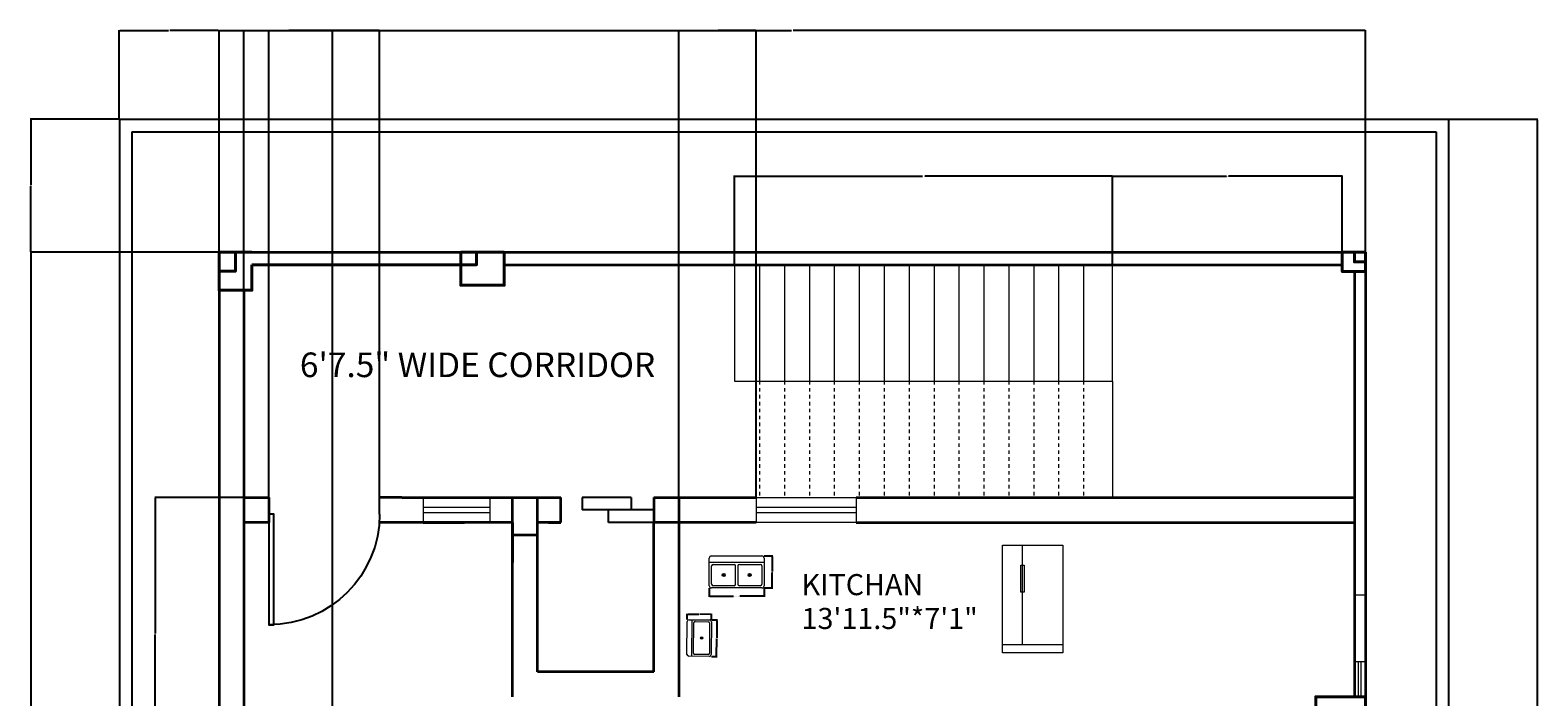
# Model space of a CAD drawing. Units: inches. Extents: x -1085 to 1941, y 1514 to 2348.
# Tile 9 of 9: x 1397 to 1941, y 1974 to 2214. Entities that reach past the tile are written whole.
import ezdxf

# ---------------------------------------------------------------- set-up
doc = ezdxf.new("R2010")
doc.units = ezdxf.units.IN
doc.linetypes.add('JIS_02_1.2', pattern=[2.5, 1.25, -1.25])
for name, color, linetype, lineweight in [('A-ANNO-DIMS', 2, 'Continuous', 18), ('A-AREA-IDEN', 7, 'Continuous', 25), ('A-COLS', 7, 'Continuous', 40), ('A-DOOR', 4, 'Continuous', 25), ('A-EQPM', 9, 'Continuous', 18), ('A-FLOR-FIXT', 9, 'Continuous', 18), ('A-FLOR-STRS', 1, 'Continuous', 18), ('A-FLOR-STRS-HIDN', 1, 'JIS_02_1.2', 18), ('A-GLAZ', 180, 'Continuous', 18), ('A-WALL', 7, 'Continuous', 35), ('C-PROP', 8, 'Continuous', 25)]:
    doc.layers.add(name, color=color, linetype=linetype, lineweight=lineweight)
doc.styles.get("Standard").update_dxf_attribs({"font": 'arial.ttf'})
doc.dimstyles.get("Standard").update_dxf_attribs({"dimtxt": 0.18, "dimasz": 0.18, "dimexe": 0.18, "dimexo": 0.0625, "dimgap": 0.09, "dimtad": 0, "dimtih": 1, "dimtoh": 1, "dimdec": 4, "dimzin": 0, "dimdsep": 46, "dimtxsty": 'Standard', "dimcen": 0.09, "dimadec": 0, "dimazin": 0, "dimtfac": 1, "dimtdec": 4, "dimtofl": 0, "dimtmove": 0, "dimatfit": 3, "dimfxl": 1, "dimtolj": 1, "dimtzin": 0, "dimarcsym": 0})

# ---------------------------------------------------------------- blocks, each defined once
blk = doc.blocks.new('*U2')
for p, q in [((0, 0), (0, -6)), ((40, 0), (40, -6))]:
    blk.add_line(p, q)
blk.add_lwpolyline([(0, 0), (0, 40), (1.75, 40), (1.75, 0)], close=True)
blk.add_arc((0, 0), 40, 0, 90)
blk = doc.blocks.new('Refrigerator-2 door - 36 in front')
for p, q in [((12, 5), (12, 64)), ((0, 5), (36, 5))]:
    blk.add_line(p, q)
for points in [[(0, 0), (0, 64), (36, 64), (36, 0)], [(11, 36), (11, 52), (13, 52), (13, 36)]]:
    blk.add_lwpolyline(points, close=True)
blk = doc.blocks.new('Sink-double - 36 in top')
for p, q in [((-18, -4), (18, -4)), ((-0.75, -18.5), (-0.75, -6.5)), ((0.75, -6.5), (0.75, -18.5))]:
    blk.add_line(p, q)
for points in [[(-16.5, 0), (16.5, 0)], [(-18, -19.5), (-18, -1.5)], [(-16.5, -18.5), (-16.5, -6.5)], [(-15.5, -5.5), (-1.75, -5.5)], [(1.75, -5.5), (15.5, -5.5)], [(16.5, -6.5), (16.5, -18.5)], [(18, -1.5), (18, -19.5)], [(-1.75, -19.5), (-15.5, -19.5)], [(15.5, -19.5), (1.75, -19.5)], [(16.5, -21), (-16.5, -21)]]:
    blk.add_lwpolyline(points)
for centre, radius in [((-8.5, -12.5), 1), ((-8.5, -12.5), 0.5), ((8.5, -12.5), 1), ((8.5, -12.5), 0.5)]:
    blk.add_circle(centre, radius)
for centre, radius, start, end in [((-16.5, -1.5), 1.5, 90, 180), ((16.5, -1.5), 1.5, 0, 90), ((-15.5, -6.5), 1, 90, 180), ((-1.75, -6.5), 1, 0, 90), ((1.75, -6.5), 1, 90, 180), ((15.5, -6.5), 1, 0, 90), ((-16.5, -19.5), 1.5, 180, 270), ((-15.5, -18.5), 1, 180, 270), ((-1.75, -18.5), 1, 270, 0), ((1.75, -18.5), 1, 180, 270), ((15.5, -18.5), 1, 270, 0), ((16.5, -19.5), 1.5, 270, 0)]:
    blk.add_arc(centre, radius, start, end)
blk = doc.blocks.new('Sink-single - 30 in top')
blk.add_line((-15, -3.999996), (15, -3.999996))
for points in [[(-13.5, 0), (13.5, 0)], [(-15, -18.499996), (-15, -1.5)], [(-13.5, -17.499996), (-13.5, -6.499996)], [(-12.5, -5.499996), (12.5, -5.499996)], [(13.5, -6.499996), (13.5, -17.499996)], [(15, -1.5), (15, -18.499996)], [(13.5, -19.999996), (-13.5, -19.999996)], [(12.5, -18.499996), (-12.5, -18.499996)]]:
    blk.add_lwpolyline(points)
for radius in [1, 0.5]:
    blk.add_circle((0, -11.999996), radius)
for centre, radius, start, end in [((-13.5, -1.5), 1.5, 90, 180), ((-12.5, -6.499996), 1, 90, 180), ((12.5, -6.499996), 1, 0, 90), ((13.5, -1.5), 1.5, 0, 90), ((-13.5, -18.499996), 1.5, 180, 270), ((-12.5, -17.499996), 1, 180, 270), ((12.5, -17.499996), 1, 270, 0), ((13.5, -18.499996), 1.5, 270, 0)]:
    blk.add_arc(centre, radius, start, end)
blk = doc.blocks.new('WIN-36-9')
for p, q in [((0, 9), (0, 0)), ((0, 5.5), (36, 5.5)), ((36, 9), (36, 0)), ((36, 3.5), (0, 3.5))]:
    blk.add_line(p, q)
blk = doc.blocks.new('*D70')
at = {"layer": 'A-ANNO-DIMS', "color": 0, "lineweight": -2, "transparency": 16777216}
for p, q in [((1642.11, 2013.01), (1642.11, 2009.92)), ((1642.29, 2010.1), (1650.92, 2010.1)), ((1661.73, 2010.1), (1653.11, 2010.1)), ((1661.91, 2013.01), (1661.91, 2009.92))]:
    blk.add_line(p, q, dxfattribs=at)
at = {"layer": 'A-ANNO-DIMS', "color": 0, "transparency": 16777216}
for points in [[(1642.29, 2010.13), (1642.29, 2010.07), (1642.11, 2010.1)], [(1661.73, 2010.13), (1661.73, 2010.07), (1661.91, 2010.1)]]:
    blk.add_solid(points, dxfattribs=at)
at = {"layer": 'Defpoints', "color": 0, "transparency": 16777216}
for p in [(1642.11, 2013.07), (1661.91, 2013.07), (1661.91, 2010.1)]:
    blk.add_point(p, dxfattribs=at)
at = {"layer": 'A-ANNO-DIMS', "color": 0, "transparency": 16777216, "insert": (1652.01, 2010.1), "char_height": 0.18, "attachment_point": 5}
blk.add_mtext('\\A1;DOUBLE SINK 20', dxfattribs=at)
blk = doc.blocks.new('*D71')
at = {"layer": 'A-ANNO-DIMS', "color": 0, "lineweight": -2, "transparency": 16777216}
for p, q in [((1661.97, 2024.62), (1665.06, 2024.62)), ((1664.88, 2024.44), (1664.88, 2019.03)), ((1664.88, 2013.25), (1664.88, 2018.67)), ((1661.97, 2013.07), (1665.06, 2013.07))]:
    blk.add_line(p, q, dxfattribs=at)
at = {"layer": 'A-ANNO-DIMS', "color": 0, "transparency": 16777216}
for points in [[(1664.85, 2024.44), (1664.91, 2024.44), (1664.88, 2024.62)], [(1664.85, 2013.25), (1664.91, 2013.25), (1664.88, 2013.07)]]:
    blk.add_solid(points, dxfattribs=at)
at = {"layer": 'Defpoints', "color": 0, "transparency": 16777216}
for p in [(1661.91, 2024.62), (1664.88, 2024.62), (1661.91, 2013.07)]:
    blk.add_point(p, dxfattribs=at)
at = {"layer": 'A-ANNO-DIMS', "color": 0, "transparency": 16777216, "insert": (1664.88, 2018.85), "char_height": 0.18, "attachment_point": 5}
blk.add_mtext('\\A1;12', dxfattribs=at)
blk = doc.blocks.new('*D72')
at = {"layer": 'A-ANNO-DIMS', "color": 0, "lineweight": -2, "transparency": 16777216}
for p, q in [((1642.98, 2001.55), (1645.08, 2001.53)), ((1644.89, 2001.36), (1644.84, 1995.13)), ((1644.78, 1988.54), (1644.84, 1994.77)), ((1642.87, 1988.38), (1644.96, 1988.36))]:
    blk.add_line(p, q, dxfattribs=at)
at = {"layer": 'A-ANNO-DIMS', "color": 0, "transparency": 16777216}
for points in [[(1644.86, 2001.36), (1644.92, 2001.36), (1644.9, 2001.54)], [(1644.75, 1988.54), (1644.81, 1988.54), (1644.78, 1988.36)]]:
    blk.add_solid(points, dxfattribs=at)
at = {"layer": 'Defpoints', "color": 0, "transparency": 16777216}
for p in [(1642.92, 2001.55), (1644.9, 2001.54), (1642.81, 1988.38)]:
    blk.add_point(p, dxfattribs=at)
at = {"layer": 'A-ANNO-DIMS', "color": 0, "transparency": 16777216, "insert": (1644.84, 1994.95), "char_height": 0.18, "attachment_point": 5}
blk.add_mtext('\\A1;SINGLE SINK 13', dxfattribs=at)
blk = doc.blocks.new('*D73')
at = {"layer": 'A-ANNO-DIMS', "color": 0, "lineweight": -2, "transparency": 16777216}
for p, q in [((1634.14, 2001.69), (1634.16, 2003.79)), ((1634.33, 2003.6), (1638.4, 2003.57)), ((1642.76, 2003.53), (1638.69, 2003.57)), ((1642.92, 2001.62), (1642.94, 2003.71))]:
    blk.add_line(p, q, dxfattribs=at)
at = {"layer": 'A-ANNO-DIMS', "color": 0, "transparency": 16777216}
for points in [[(1634.33, 2003.63), (1634.33, 2003.57), (1634.15, 2003.61)], [(1642.76, 2003.56), (1642.76, 2003.5), (1642.94, 2003.53)]]:
    blk.add_solid(points, dxfattribs=at)
at = {"layer": 'Defpoints', "color": 0, "transparency": 16777216}
for p in [(1634.15, 2003.61), (1634.14, 2001.63), (1642.92, 2001.55)]:
    blk.add_point(p, dxfattribs=at)
at = {"layer": 'A-ANNO-DIMS', "color": 0, "transparency": 16777216, "insert": (1638.55, 2003.57), "char_height": 0.18, "attachment_point": 5}
blk.add_mtext('\\A1;9', dxfattribs=at)
blk = doc.blocks.new('*D75')
at = {"layer": 'A-ANNO-DIMS', "color": 0, "lineweight": -2, "transparency": 16777216}
for p, q in [((1909.16, 2182.24), (1941.27, 2182.24)), ((1941.09, 2182.06), (1941.09, 1864.42)), ((1941.09, 1546.42), (1941.09, 1864.06)), ((1909.16, 1546.24), (1941.27, 1546.24))]:
    blk.add_line(p, q, dxfattribs=at)
at = {"layer": 'A-ANNO-DIMS', "color": 0, "transparency": 16777216}
for points in [[(1941.06, 2182.06), (1941.12, 2182.06), (1941.09, 2182.24)], [(1941.06, 1546.42), (1941.12, 1546.42), (1941.09, 1546.24)]]:
    blk.add_solid(points, dxfattribs=at)
at = {"layer": 'Defpoints', "color": 0, "transparency": 16777216}
for p in [(1909.09, 2182.24), (1941.09, 2182.24), (1909.09, 1546.24)]:
    blk.add_point(p, dxfattribs=at)
at = {"layer": 'A-ANNO-DIMS', "color": 0, "transparency": 16777216, "insert": (1941.09, 1864.24), "char_height": 0.18, "attachment_point": 5}
blk.add_mtext('\\A1;636', dxfattribs=at)
blk = doc.blocks.new('*D76')
at = {"layer": 'A-ANNO-DIMS', "color": 0, "lineweight": -2, "transparency": 16777216}
for p, q in [((1465.09, 2134.3), (1465.09, 2214.42)), ((1465.27, 2214.24), (1671.8, 2214.24)), ((1878.91, 2214.24), (1672.39, 2214.24)), ((1879.09, 2134.3), (1879.09, 2214.42))]:
    blk.add_line(p, q, dxfattribs=at)
at = {"layer": 'A-ANNO-DIMS', "color": 0, "transparency": 16777216}
for points in [[(1465.27, 2214.27), (1465.27, 2214.21), (1465.09, 2214.24)], [(1878.91, 2214.27), (1878.91, 2214.21), (1879.09, 2214.24)]]:
    blk.add_solid(points, dxfattribs=at)
at = {"layer": 'Defpoints', "color": 0, "transparency": 16777216}
for p in [(1879.09, 2214.24), (1465.09, 2134.24), (1879.09, 2134.24)]:
    blk.add_point(p, dxfattribs=at)
at = {"layer": 'A-ANNO-DIMS', "color": 0, "transparency": 16777216, "insert": (1672.09, 2214.24), "char_height": 0.18, "attachment_point": 5}
blk.add_mtext('\\A1;414', dxfattribs=at)
blk = doc.blocks.new('*D77')
at = {"layer": 'A-ANNO-DIMS', "color": 0, "lineweight": -2, "transparency": 16777216}
for p, q in [((1465.03, 2134.24), (1396.91, 2134.24)), ((1397.09, 2134.06), (1397.09, 1855.42)), ((1397.09, 1576.42), (1397.09, 1855.06)), ((1465.03, 1576.24), (1396.91, 1576.24))]:
    blk.add_line(p, q, dxfattribs=at)
at = {"layer": 'A-ANNO-DIMS', "color": 0, "transparency": 16777216}
for points in [[(1397.06, 2134.06), (1397.12, 2134.06), (1397.09, 2134.24)], [(1397.06, 1576.42), (1397.12, 1576.42), (1397.09, 1576.24)]]:
    blk.add_solid(points, dxfattribs=at)
at = {"layer": 'Defpoints', "color": 0, "transparency": 16777216}
for p in [(1397.09, 2134.24), (1465.09, 2134.24), (1465.09, 1576.24)]:
    blk.add_point(p, dxfattribs=at)
at = {"layer": 'A-ANNO-DIMS', "color": 0, "transparency": 16777216, "insert": (1397.09, 1855.24), "char_height": 0.18, "attachment_point": 5}
blk.add_mtext('\\A1;558', dxfattribs=at)
blk = doc.blocks.new('*D78')
at = {"layer": 'A-ANNO-DIMS', "color": 0, "lineweight": -2, "transparency": 16777216}
for p, q in [((1429.09, 2182.3), (1429.09, 2214.42)), ((1429.27, 2214.24), (1446.88, 2214.24)), ((1464.91, 2214.24), (1447.31, 2214.24)), ((1465.09, 2134.3), (1465.09, 2214.42))]:
    blk.add_line(p, q, dxfattribs=at)
at = {"layer": 'A-ANNO-DIMS', "color": 0, "transparency": 16777216}
for points in [[(1429.27, 2214.27), (1429.27, 2214.21), (1429.09, 2214.24)], [(1464.91, 2214.27), (1464.91, 2214.21), (1465.09, 2214.24)]]:
    blk.add_solid(points, dxfattribs=at)
at = {"layer": 'Defpoints', "color": 0, "transparency": 16777216}
for p in [(1465.09, 2214.24), (1429.09, 2182.24), (1465.09, 2134.24)]:
    blk.add_point(p, dxfattribs=at)
at = {"layer": 'A-ANNO-DIMS', "color": 0, "transparency": 16777216, "insert": (1447.09, 2214.24), "char_height": 0.18, "attachment_point": 5}
blk.add_mtext('\\A1;36', dxfattribs=at)
blk = doc.blocks.new('*D79')
at = {"layer": 'A-ANNO-DIMS', "color": 0, "lineweight": -2, "transparency": 16777216}
for p, q in [((1429.03, 2182.24), (1396.91, 2182.24)), ((1397.09, 2182.06), (1397.09, 2158.42)), ((1397.09, 2134.42), (1397.09, 2158.06)), ((1465.03, 2134.24), (1396.91, 2134.24))]:
    blk.add_line(p, q, dxfattribs=at)
at = {"layer": 'A-ANNO-DIMS', "color": 0, "transparency": 16777216}
for points in [[(1397.06, 2182.06), (1397.12, 2182.06), (1397.09, 2182.24)], [(1397.06, 2134.42), (1397.12, 2134.42), (1397.09, 2134.24)]]:
    blk.add_solid(points, dxfattribs=at)
at = {"layer": 'Defpoints', "color": 0, "transparency": 16777216}
for p in [(1429.09, 2182.24), (1397.09, 2134.24), (1465.09, 2134.24)]:
    blk.add_point(p, dxfattribs=at)
at = {"layer": 'A-ANNO-DIMS', "color": 0, "transparency": 16777216, "insert": (1397.09, 2158.24), "char_height": 0.18, "attachment_point": 5}
blk.add_mtext('\\A1;48', dxfattribs=at)
blk = doc.blocks.new('*D80')
at = {"layer": 'A-ANNO-DIMS', "color": 0, "lineweight": -2, "transparency": 16777216}
for p, q in [((1483.09, 2045.8), (1483.09, 2214.42)), ((1483.27, 2214.24), (1502.87, 2214.24)), ((1522.91, 2214.24), (1503.32, 2214.24)), ((1523.09, 2045.8), (1523.09, 2214.42))]:
    blk.add_line(p, q, dxfattribs=at)
at = {"layer": 'A-ANNO-DIMS', "color": 0, "transparency": 16777216}
for points in [[(1483.27, 2214.27), (1483.27, 2214.21), (1483.09, 2214.24)], [(1522.91, 2214.27), (1522.91, 2214.21), (1523.09, 2214.24)]]:
    blk.add_solid(points, dxfattribs=at)
at = {"layer": 'Defpoints', "color": 0, "transparency": 16777216}
for p in [(1523.09, 2214.24), (1483.09, 2045.74), (1523.09, 2045.74)]:
    blk.add_point(p, dxfattribs=at)
at = {"layer": 'A-ANNO-DIMS', "color": 0, "transparency": 16777216, "insert": (1503.09, 2214.24), "char_height": 0.18, "attachment_point": 5}
blk.add_mtext('\\A1;40', dxfattribs=at)
blk = doc.blocks.new('*D84')
at = {"layer": 'A-ANNO-DIMS', "color": 0, "lineweight": -2, "transparency": 16777216}
for p, q in [((1474.09, 1651.3), (1474.09, 2214.42)), ((1474.27, 2214.24), (1489.88, 2214.24)), ((1505.91, 2214.24), (1490.31, 2214.24)), ((1506.09, 1651.3), (1506.09, 2214.42))]:
    blk.add_line(p, q, dxfattribs=at)
at = {"layer": 'A-ANNO-DIMS', "color": 0, "transparency": 16777216}
for points in [[(1474.27, 2214.27), (1474.27, 2214.21), (1474.09, 2214.24)], [(1505.91, 2214.27), (1505.91, 2214.21), (1506.09, 2214.24)]]:
    blk.add_solid(points, dxfattribs=at)
at = {"layer": 'Defpoints', "color": 0, "transparency": 16777216}
for p in [(1506.09, 2214.24), (1474.09, 1651.24), (1506.09, 1651.24)]:
    blk.add_point(p, dxfattribs=at)
at = {"layer": 'A-ANNO-DIMS', "color": 0, "transparency": 16777216, "insert": (1490.09, 2214.24), "char_height": 0.18, "attachment_point": 5}
blk.add_mtext('\\A1;32', dxfattribs=at)
blk = doc.blocks.new('*D90')
at = {"layer": 'A-ANNO-DIMS', "color": 0, "lineweight": -2, "transparency": 16777216}
for p, q in [((1474.03, 2045.74), (1441.91, 2045.74)), ((1442.09, 2045.56), (1442.09, 1996.67)), ((1442.09, 1947.42), (1442.09, 1996.31)), ((1474.03, 1947.24), (1441.91, 1947.24))]:
    blk.add_line(p, q, dxfattribs=at)
at = {"layer": 'A-ANNO-DIMS', "color": 0, "transparency": 16777216}
for points in [[(1442.06, 2045.56), (1442.12, 2045.56), (1442.09, 2045.74)], [(1442.06, 1947.42), (1442.12, 1947.42), (1442.09, 1947.24)]]:
    blk.add_solid(points, dxfattribs=at)
at = {"layer": 'Defpoints', "color": 0, "transparency": 16777216}
for p in [(1442.09, 2045.74), (1474.09, 2045.74), (1474.09, 1947.24)]:
    blk.add_point(p, dxfattribs=at)
at = {"layer": 'A-ANNO-DIMS', "color": 0, "transparency": 16777216, "insert": (1442.09, 1996.49), "char_height": 0.18, "attachment_point": 5}
blk.add_mtext('\\A1;98.5', dxfattribs=at)
blk = doc.blocks.new('*D91')
at = {"layer": 'A-ANNO-DIMS', "color": 0, "lineweight": -2, "transparency": 16777216}
for p, q in [((1631.09, 2045.8), (1631.09, 2214.42)), ((1631.27, 2214.24), (1644.87, 2214.24)), ((1658.91, 2214.24), (1645.32, 2214.24)), ((1659.09, 2045.8), (1659.09, 2214.42))]:
    blk.add_line(p, q, dxfattribs=at)
at = {"layer": 'A-ANNO-DIMS', "color": 0, "transparency": 16777216}
for points in [[(1631.27, 2214.27), (1631.27, 2214.21), (1631.09, 2214.24)], [(1658.91, 2214.27), (1658.91, 2214.21), (1659.09, 2214.24)]]:
    blk.add_solid(points, dxfattribs=at)
at = {"layer": 'Defpoints', "color": 0, "transparency": 16777216}
for p in [(1659.09, 2214.24), (1631.09, 2045.74), (1659.09, 2045.74)]:
    blk.add_point(p, dxfattribs=at)
at = {"layer": 'A-ANNO-DIMS', "color": 0, "transparency": 16777216, "insert": (1645.09, 2214.24), "char_height": 0.18, "attachment_point": 5}
blk.add_mtext('\\A1;28', dxfattribs=at)
blk = doc.blocks.new('*D92')
at = {"layer": 'A-ANNO-DIMS', "color": 0, "lineweight": -2, "transparency": 16777216}
for p, q in [((1651.26, 2129.8), (1651.26, 2161.92)), ((1651.44, 2161.74), (1719.05, 2161.74)), ((1787.57, 2161.74), (1719.96, 2161.74)), ((1787.75, 2129.8), (1787.75, 2161.92))]:
    blk.add_line(p, q, dxfattribs=at)
at = {"layer": 'A-ANNO-DIMS', "color": 0, "transparency": 16777216}
for points in [[(1651.44, 2161.77), (1651.44, 2161.71), (1651.26, 2161.74)], [(1787.57, 2161.77), (1787.57, 2161.71), (1787.75, 2161.74)]]:
    blk.add_solid(points, dxfattribs=at)
at = {"layer": 'Defpoints', "color": 0, "transparency": 16777216}
for p in [(1787.75, 2161.74), (1651.26, 2129.74), (1787.75, 2129.74)]:
    blk.add_point(p, dxfattribs=at)
at = {"layer": 'A-ANNO-DIMS', "color": 0, "transparency": 16777216, "insert": (1719.5, 2161.74), "char_height": 0.18, "attachment_point": 5}
blk.add_mtext('\\A1;136.48', dxfattribs=at)
blk = doc.blocks.new('*D93')
at = {"layer": 'A-ANNO-DIMS', "color": 0, "lineweight": -2, "transparency": 16777216}
for p, q in [((1787.75, 2129.8), (1787.75, 2161.92)), ((1787.93, 2161.74), (1828.82, 2161.74)), ((1870.5, 2161.74), (1829.61, 2161.74)), ((1870.68, 2129.8), (1870.68, 2161.92))]:
    blk.add_line(p, q, dxfattribs=at)
at = {"layer": 'A-ANNO-DIMS', "color": 0, "transparency": 16777216}
for points in [[(1787.93, 2161.77), (1787.93, 2161.71), (1787.75, 2161.74)], [(1870.5, 2161.77), (1870.5, 2161.71), (1870.68, 2161.74)]]:
    blk.add_solid(points, dxfattribs=at)
at = {"layer": 'Defpoints', "color": 0, "transparency": 16777216}
for p in [(1870.68, 2161.74), (1787.75, 2129.74), (1870.68, 2129.74)]:
    blk.add_point(p, dxfattribs=at)
at = {"layer": 'A-ANNO-DIMS', "color": 0, "transparency": 16777216, "insert": (1829.21, 2161.74), "char_height": 0.18, "attachment_point": 5}
blk.add_mtext('\\A1;82.93', dxfattribs=at)

msp = doc.modelspace()

# ---------------------------------------------------------------- linework, layer by layer
at = {"layer": 'A-COLS'}
msp.add_lwpolyline([(1476.9484, 2129.7392), (1476.9484, 2120.553), (1465.0949, 2120.553), (1465.0949, 2134.2392), (1476.9484, 2134.2392)], dxfattribs=at)
for points in [[(1465.0949, 2134.2392), (1471.0216, 2134.2392), (1471.0216, 2127.3961), (1465.0949, 2127.3961)], [(1552.4003, 2134.2392), (1568.1037, 2134.2392), (1568.1037, 2122.3334), (1552.4003, 2122.3334)], [(1552.4003, 2134.2392), (1558.0949, 2134.2392), (1558.0949, 2129.7392), (1552.4003, 2129.7392)], [(1879.0949, 2134.2392), (1870.6776, 2134.2392), (1870.6776, 2127.2968), (1879.0949, 2127.2968)], [(1879.0949, 2134.2392), (1875.0637, 2134.2392), (1875.0637, 2130.768), (1879.0949, 2130.768)], [(1879.0949, 1973.8073), (1879.0949, 1961.8073), (1861.0949, 1961.8073), (1861.0949, 1973.8073)]]:
    msp.add_lwpolyline(points, close=True, dxfattribs=at)
at = {"layer": 'A-DOOR'}
for p, q in [((1613.8856, 2045.7392), (1596.2389, 2045.7392)), ((1596.2389, 2045.7392), (1596.2389, 2041.2392)), ((1613.8856, 2045.7392), (1613.8856, 2041.2392)), ((1613.8856, 2041.2392), (1596.2389, 2041.2392)), ((1622.0949, 2041.2392), (1605.6763, 2041.2392)), ((1605.6763, 2036.7392), (1605.6763, 2041.2392)), ((1622.0949, 2036.7392), (1605.6763, 2036.7392))]:
    msp.add_line(p, q, dxfattribs=at)
at = {"layer": 'A-FLOR-STRS'}
for p, q in [((1651.2617, 2129.7392), (1651.2617, 2087.7392)), ((1660.2617, 2129.7392), (1660.2617, 2087.7392)), ((1669.2617, 2129.7392), (1669.2617, 2087.7392)), ((1678.2617, 2129.7392), (1678.2617, 2087.7392)), ((1687.2617, 2129.7392), (1687.2617, 2087.7392)), ((1696.2617, 2129.7392), (1696.2617, 2087.7392)), ((1705.2617, 2129.7392), (1705.2617, 2087.7392)), ((1714.2617, 2129.7392), (1714.2617, 2087.7392)), ((1723.2617, 2129.7392), (1723.2617, 2087.7392)), ((1732.2617, 2129.7392), (1732.2617, 2087.7392)), ((1741.2617, 2129.7392), (1741.2617, 2087.7392)), ((1750.2617, 2129.7392), (1750.2617, 2087.7392)), ((1759.2617, 2129.7392), (1759.2617, 2087.7392)), ((1768.2617, 2129.7392), (1768.2617, 2087.7392)), ((1777.2617, 2129.7392), (1777.2617, 2087.7392)), ((1787.7455, 2087.7392), (1787.7455, 2129.7392)), ((1651.2617, 2087.7392), (1787.7455, 2087.7392)), ((1787.7455, 2087.7392), (1787.7455, 2045.7392))]:
    msp.add_line(p, q, dxfattribs=at)
at = {"layer": 'A-FLOR-STRS-HIDN'}
for p, q in [((1660.2617, 2087.7392), (1660.2617, 2045.7392)), ((1669.2617, 2087.7392), (1669.2617, 2045.7392)), ((1678.2617, 2087.7392), (1678.2617, 2045.7392)), ((1687.2617, 2087.7392), (1687.2617, 2045.7392)), ((1696.2617, 2087.7392), (1696.2617, 2045.7392)), ((1705.2617, 2087.7392), (1705.2617, 2045.7392)), ((1705.2617, 2087.7392), (1705.2617, 2045.7392)), ((1714.2617, 2087.7392), (1714.2617, 2045.7392)), ((1723.2617, 2087.7392), (1723.2617, 2045.7392)), ((1732.2617, 2087.7392), (1732.2617, 2045.7392)), ((1741.2617, 2087.7392), (1741.2617, 2045.7392)), ((1750.2617, 2087.7392), (1750.2617, 2045.7392)), ((1759.2617, 2087.7392), (1759.2617, 2045.7392)), ((1768.2617, 2087.7392), (1768.2617, 2045.7392)), ((1777.2617, 2087.7392), (1777.2617, 2045.7392))]:
    msp.add_line(p, q, dxfattribs=at)
at = {"layer": 'A-GLAZ'}
for p, q in [((1538.837, 2045.7392), (1538.837, 2036.7392)), ((1538.837, 2042.2392), (1552.5949, 2042.2392)), ((1552.5949, 2042.2392), (1562.837, 2042.2392)), ((1562.837, 2045.7392), (1562.837, 2036.7392)), ((1659.0949, 2045.7392), (1695.0949, 2045.7392)), ((1552.5949, 2040.2392), (1538.837, 2040.2392)), ((1562.837, 2040.2392), (1552.5949, 2040.2392)), ((1695.0949, 2036.7392), (1659.0949, 2036.7392)), ((1875.0637, 2010.5526), (1879.0949, 2010.5526)), ((1875.0637, 1986.5526), (1879.0949, 1986.5526)), ((1876.578, 1973.8073), (1876.578, 1986.5526)), ((1877.5219, 1973.8073), (1877.5219, 1986.5526))]:
    msp.add_line(p, q, dxfattribs=at)
at = {"layer": 'A-WALL'}
for p, q in [((1465.0949, 2134.2392), (1879.0949, 2134.2392)), ((1465.0949, 2134.2392), (1465.0949, 1576.2392)), ((1879.0949, 2134.2392), (1879.0949, 1576.2392)), ((1474.0949, 2129.7392), (1474.0949, 2129.7392)), ((1476.9484, 2129.7392), (1558.0949, 2129.7392)), ((1476.9484, 2129.7392), (1558.0949, 2129.7392)), ((1558.0949, 2129.7392), (1476.9484, 2129.7392)), ((1476.9484, 2129.7392), (1558.0949, 2129.7392)), ((1568.1037, 2129.7392), (1584.6191, 2129.7392)), ((1568.1037, 2129.7392), (1870.6776, 2129.7392)), ((1875.0637, 2127.2968), (1875.0637, 1973.8073)), ((1474.0949, 2120.553), (1474.0949, 1585.4303)), ((1474.0949, 2120.553), (1474.0949, 2045.7392)), ((1474.0949, 2045.7392), (1483.0949, 2045.7392)), ((1483.0949, 2045.7392), (1483.0949, 2036.7392)), ((1531.0949, 2045.7392), (1523.0949, 2045.7392)), ((1531.0949, 2045.7392), (1552.5949, 2045.7392)), ((1552.5949, 2045.7392), (1588.5036, 2045.7392)), ((1571.0949, 2036.7392), (1571.0949, 2045.7392)), ((1580.0949, 2036.7392), (1580.0949, 2045.7392)), ((1588.5036, 2036.7392), (1588.5036, 2045.7392)), ((1622.0949, 2045.7392), (1622.0949, 2036.7392)), ((1622.0949, 2045.7392), (1631.0949, 2045.7392)), ((1631.0949, 2045.7392), (1631.0949, 2036.7392)), ((1631.0949, 2045.7392), (1659.0949, 2045.7392)), ((1695.0949, 2045.7392), (1875.0637, 2045.7392)), ((1483.0949, 2036.7392), (1474.0949, 2036.7392)), ((1538.837, 2036.7392), (1522.9822, 2036.7392)), ((1538.837, 2036.7392), (1553.6692, 2036.7392)), ((1553.6692, 2036.7392), (1538.837, 2036.7392)), ((1571.0949, 2036.7392), (1552.5949, 2036.7392)), ((1571.0949, 1973.7392), (1571.0949, 2036.7392)), ((1571.0949, 2036.7392), (1571.0949, 2022.2616)), ((1588.5036, 2036.7392), (1580.0949, 2036.7392)), ((1580.0949, 1982.7392), (1580.0949, 2036.7392)), ((1584.0527, 2036.7392), (1584.0527, 2036.7392)), ((1584.0527, 2036.7392), (1588.5036, 2036.7392)), ((1631.0949, 2036.7392), (1622.0949, 2036.7392)), ((1622.0949, 1982.7392), (1622.0949, 2036.7392)), ((1631.0949, 2036.7392), (1631.0949, 1973.7392)), ((1659.0949, 2036.7392), (1631.0949, 2036.7392)), ((1695.0949, 2036.7392), (1875.0637, 2036.7392)), ((1571.0949, 2032.245), (1580.0949, 2032.245)), ((1622.0949, 1982.7392), (1580.0949, 1982.7392))]:
    msp.add_line(p, q, dxfattribs=at)
at = {"layer": 'C-PROP'}
for p, q in [((1429.0949, 2182.2392), (1909.0949, 2182.2392)), ((1429.0949, 2182.2392), (1429.0949, 1546.2392)), ((1433.5949, 2177.7392), (1904.5949, 2177.7392)), ((1433.5949, 2177.7392), (1433.5949, 1550.7392)), ((1904.5949, 2177.7392), (1904.5949, 1550.7392)), ((1909.0949, 2182.2392), (1909.0949, 1546.2392))]:
    msp.add_line(p, q, dxfattribs=at)

# ---------------------------------------------------------------- block references
at = {"layer": 'A-DOOR', "xscale": -1, "rotation": 180}
msp.add_blockref('*U2', (1483.0949, 2039.7392), dxfattribs=at)
at = {"layer": 'A-EQPM', "xscale": 0.6082930186288423, "yscale": 0.6082930186288423, "zscale": 0.6082930186288423}
msp.add_blockref('Refrigerator-2 door - 36 in front', (1747.9351, 1989.639), dxfattribs=at)
at = {"layer": 'A-FLOR-FIXT', "xscale": 0.5499719409228704, "yscale": 0.5499719409228704, "zscale": 0.5499719409228704}
msp.add_blockref('Sink-double - 36 in top', (1652.0117, 2024.6228), dxfattribs=at)
at = {"layer": 'A-FLOR-FIXT', "xscale": 0.4391326192988868, "yscale": 0.4391326192988868, "zscale": 0.4391326192988868, "rotation": 89.50221043025716}
msp.add_blockref('Sink-single - 30 in top', (1634.0802, 1995.0429), dxfattribs=at)
at = {"layer": 'A-GLAZ'}
msp.add_blockref('WIN-36-9', (1659.095, 2036.739), dxfattribs=at)

# ---------------------------------------------------------------- texts
at = {"layer": 'A-ANNO-DIMS'}
msp.add_text('13\'11.5"*7\'1"', height=7.604031, dxfattribs=at).set_placement((1675.4369, 1998.2564))
at = {"layer": 'A-AREA-IDEN'}
for s, height, p in [('6\'7.5" WIDE CORRIDOR', 8.873974, (1494.2857, 2089.1831)), ('KITCHAN', 7.60403, (1675.4369, 2010.4717))]:
    msp.add_text(s, height=height, dxfattribs=at).set_placement(p)

# ---------------------------------------------------------------- dimensions: what is measured, and where the dimension line sits
at = {"layer": 'A-ANNO-DIMS'}
for base, p1, p2, override, picture, middle in [((1465.0949, 2214.2392), (1429.0949, 2182.2392), (1465.0949, 2134.2392), {"dimdec": 0, "dimlfac": 1, "dimrnd": 0, "dimzin": 0, "dimdsep": 46, "dimlunit": 2}, '*D78', (1447.0949, 2214.2392)), ((1879.0949, 2214.2392), (1465.0949, 2134.2392), (1879.0949, 2134.2392), {"dimdec": 0, "dimlfac": 1, "dimrnd": 0, "dimzin": 0, "dimdsep": 46, "dimlunit": 2}, '*D76', (1672.0949, 2214.2392)), ((1506.0949, 2214.2392), (1474.0949, 1651.2392), (1506.0949, 1651.2392), {"dimdec": 0, "dimlfac": 1, "dimrnd": 0, "dimzin": 0, "dimdsep": 46, "dimlunit": 2}, '*D84', (1490.0949, 2214.2392)), ((1523.0949, 2214.2392), (1483.0949, 2045.7392), (1523.0949, 2045.7392), {"dimdec": 0, "dimlfac": 1, "dimrnd": 0, "dimzin": 0, "dimdsep": 46, "dimlunit": 2}, '*D80', (1503.0949, 2214.2392)), ((1659.0949, 2214.2392), (1631.0949, 2045.7392), (1659.0949, 2045.7392), {"dimdec": 0, "dimlfac": 1, "dimrnd": 0, "dimzin": 0, "dimdsep": 46, "dimlunit": 2}, '*D91', (1645.0949, 2214.2392)), ((1787.7455, 2161.7392), (1651.2617, 2129.7392), (1787.7455, 2129.7392), {"dimdec": 2, "dimlfac": 1, "dimrnd": 0, "dimzin": 0, "dimdsep": 46, "dimlunit": 2}, '*D92', (1719.5036, 2161.7392)), ((1870.6776, 2161.7392), (1787.7455, 2129.7392), (1870.6776, 2129.7392), {"dimdec": 2, "dimlfac": 1, "dimrnd": 0, "dimzin": 0, "dimdsep": 46, "dimlunit": 2}, '*D93', (1829.2116, 2161.7392))]:
    dim = msp.add_linear_dim(base=base, p1=p1, p2=p2, dimstyle='Standard', override=override, dxfattribs=at)
    dim.commit()
    dim.dimension.update_dxf_attribs({"geometry": picture, "text_midpoint": middle})
for base, p1, p2, angle, override, picture, middle in [((1397.0949, 2134.2392), (1429.0949, 2182.2392), (1465.0949, 2134.2392), 90, {"dimdec": 0, "dimlfac": 1, "dimrnd": 0, "dimzin": 0, "dimdsep": 46, "dimlunit": 2}, '*D79', (1397.0949, 2158.2392)), ((1941.0949, 2182.2392), (1909.0949, 1546.2392), (1909.0949, 2182.2392), 90, {"dimdec": 0, "dimlfac": 1, "dimrnd": 0, "dimzin": 0, "dimdsep": 46, "dimlunit": 2}, '*D75', (1941.0949, 1864.2392)), ((1397.0949, 2134.2392), (1465.0949, 1576.2392), (1465.0949, 2134.2392), 90, {"dimdec": 0, "dimlfac": 1, "dimrnd": 0, "dimzin": 0, "dimdsep": 46, "dimlunit": 2}, '*D77', (1397.0949, 1855.2392)), ((1442.0949, 2045.7392), (1474.0949, 1947.2392), (1474.0949, 2045.7392), 90, {"dimdec": 1, "dimlfac": 1, "dimrnd": 0, "dimzin": 0, "dimdsep": 46, "dimlunit": 2}, '*D90', (1442.0949, 1996.4892)), ((1664.881, 2024.6228), (1661.9112, 2013.0734), (1661.9112, 2024.6228), 90, {"dimdec": 0, "dimlfac": 1, "dimrnd": 0, "dimzin": 0, "dimdsep": 46, "dimlunit": 2}, '*D71', (1664.881, 2018.8481)), ((1634.1546, 2003.6057), (1642.9197, 2001.5533), (1634.1374, 2001.6296), 179.50221, {"dimdec": 0, "dimlfac": 1, "dimrnd": 0, "dimzin": 0, "dimdsep": 46, "dimlunit": 2}, '*D73', (1638.5457, 2003.5675))]:
    dim = msp.add_linear_dim(base=base, p1=p1, p2=p2, angle=angle, dimstyle='Standard', override=override, dxfattribs=at)
    dim.commit()
    dim.dimension.update_dxf_attribs({"geometry": picture, "text_midpoint": middle})
dim = msp.add_linear_dim(base=(1661.9112, 2010.1035), p1=(1642.1122, 2013.0734), p2=(1661.9112, 2013.0734), text='DOUBLE SINK <>', dimstyle='Standard', override={"dimdec": 0, "dimlfac": 1, "dimrnd": 0, "dimzin": 0, "dimdsep": 46, "dimlunit": 2}, dxfattribs=at)
dim.commit()
dim.dimension.update_dxf_attribs({"geometry": '*D70', "text_midpoint": (1652.0117, 2010.1035)})
dim = msp.add_linear_dim(base=(1644.8958, 2001.5362), p1=(1642.8053, 1988.3799), p2=(1642.9197, 2001.5533), angle=89.50221, text='SINGLE SINK <>', dimstyle='Standard', override={"dimdec": 0, "dimlfac": 1, "dimrnd": 0, "dimzin": 0, "dimdsep": 46, "dimlunit": 2}, dxfattribs=at)
dim.commit()
dim.dimension.update_dxf_attribs({"geometry": '*D72', "text_midpoint": (1644.8385, 1994.9494)})

doc.saveas('drawing.dxf')
